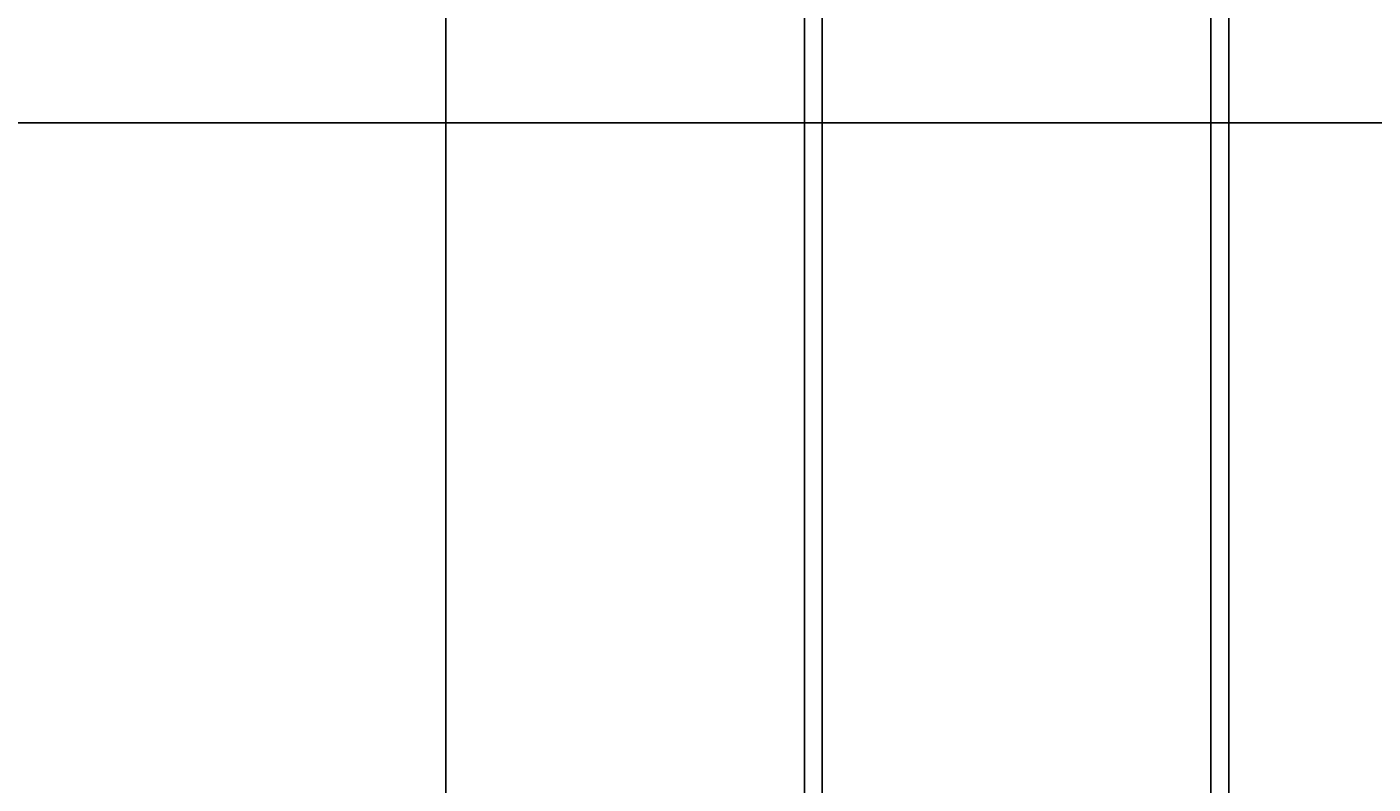
# Model space of a CAD drawing. Units: inches. Extents: x 1770 to 2988, y 1161 to 3221.
# Tile 19 of 44: x 2090 to 2289, y 2409 to 2520. Entities that reach past the tile are written whole.
import ezdxf

# ---------------------------------------------------------------- set-up
doc = ezdxf.new("R2010")
doc.units = ezdxf.units.IN
doc.layers.add('A-ANNO-DIMS', color=2, linetype='Continuous', lineweight=18)
doc.layers.add('C-PROP', color=7, linetype='Continuous', lineweight=25)
doc.styles.get("Standard").update_dxf_attribs({"font": 'arial.ttf'})
doc.dimstyles.get("Standard").update_dxf_attribs({"dimtxt": 0.18, "dimasz": 0.18, "dimexe": 0.18, "dimexo": 0.0625, "dimgap": 0.09, "dimtad": 0, "dimtih": 1, "dimtoh": 1, "dimdec": 4, "dimzin": 0, "dimdsep": 46, "dimtxsty": 'Standard', "dimcen": 0.09, "dimadec": 0, "dimazin": 0, "dimtfac": 1, "dimtdec": 4, "dimtofl": 0, "dimtmove": 0, "dimatfit": 3, "dimfxl": 1, "dimtolj": 1, "dimtzin": 0, "dimarcsym": 0})

# ---------------------------------------------------------------- blocks, each defined once
blk = doc.blocks.new('*D56')
at = {"layer": 'A-ANNO-DIMS', "color": 0, "lineweight": -2, "transparency": 16777216}
for p, q in [((1971.53, 2506.34), (1971.53, 2570.7)), ((1971.71, 2570.52), (2386.59, 2570.52)), ((2802.26, 2570.52), (2387.38, 2570.52)), ((2802.44, 2506.34), (2802.44, 2570.7))]:
    blk.add_line(p, q, dxfattribs=at)
at = {"layer": 'A-ANNO-DIMS', "color": 0, "transparency": 16777216}
for points in [[(1971.71, 2570.55), (1971.71, 2570.49), (1971.53, 2570.52)], [(2802.26, 2570.55), (2802.26, 2570.49), (2802.44, 2570.52)]]:
    blk.add_solid(points, dxfattribs=at)
at = {"layer": 'Defpoints', "color": 0, "transparency": 16777216}
for p in [(2802.44, 2570.52), (1971.53, 2506.27), (2802.44, 2506.27)]:
    blk.add_point(p, dxfattribs=at)
at = {"layer": 'A-ANNO-DIMS', "color": 0, "transparency": 16777216, "insert": (2386.99, 2570.52), "char_height": 0.18, "attachment_point": 5}
blk.add_mtext('\\A1;830.9', dxfattribs=at)
blk = doc.blocks.new('*D64')
at = {"layer": 'A-ANNO-DIMS', "color": 0, "lineweight": -2, "transparency": 16777216}
for p, q in [((2151.7, 2376.76), (2151.7, 2570.7)), ((2151.88, 2570.52), (2179.09, 2570.52)), ((2207.1, 2570.52), (2179.88, 2570.52)), ((2207.28, 2376.76), (2207.28, 2570.7))]:
    blk.add_line(p, q, dxfattribs=at)
at = {"layer": 'A-ANNO-DIMS', "color": 0, "transparency": 16777216}
for points in [[(2151.88, 2570.55), (2151.88, 2570.49), (2151.7, 2570.52)], [(2207.1, 2570.55), (2207.1, 2570.49), (2207.28, 2570.52)]]:
    blk.add_solid(points, dxfattribs=at)
at = {"layer": 'Defpoints', "color": 0, "transparency": 16777216}
for p in [(2207.28, 2570.52), (2151.7, 2376.7), (2207.28, 2376.7)]:
    blk.add_point(p, dxfattribs=at)
at = {"layer": 'A-ANNO-DIMS', "color": 0, "transparency": 16777216, "insert": (2179.49, 2570.52), "char_height": 0.18, "attachment_point": 5}
blk.add_mtext('\\A1;55.58', dxfattribs=at)
blk = doc.blocks.new('*D65')
at = {"layer": 'A-ANNO-DIMS', "color": 0, "lineweight": -2, "transparency": 16777216}
for p, q in [((2267.28, 2376.76), (2267.28, 2570.7)), ((2267.46, 2570.52), (2320.24, 2570.52)), ((2373.79, 2570.52), (2321.01, 2570.52)), ((2373.97, 2376.76), (2373.97, 2570.7))]:
    blk.add_line(p, q, dxfattribs=at)
at = {"layer": 'A-ANNO-DIMS', "color": 0, "transparency": 16777216}
for points in [[(2267.46, 2570.55), (2267.46, 2570.49), (2267.28, 2570.52)], [(2373.79, 2570.55), (2373.79, 2570.49), (2373.97, 2570.52)]]:
    blk.add_solid(points, dxfattribs=at)
at = {"layer": 'Defpoints', "color": 0, "transparency": 16777216}
for p in [(2373.97, 2570.52), (2267.28, 2376.7), (2373.97, 2376.7)]:
    blk.add_point(p, dxfattribs=at)
at = {"layer": 'A-ANNO-DIMS', "color": 0, "transparency": 16777216, "insert": (2320.62, 2570.52), "char_height": 0.18, "attachment_point": 5}
blk.add_mtext('\\A1;106.7', dxfattribs=at)
blk = doc.blocks.new('*D79')
at = {"layer": 'A-ANNO-DIMS', "color": 0, "lineweight": -2, "transparency": 16777216}
for p, q in [((2151.7, 1610.26), (2151.7, 2570.7)), ((2151.88, 2570.52), (2177.78, 2570.52)), ((2204.48, 2570.52), (2178.57, 2570.52)), ((2204.66, 1610.26), (2204.66, 2570.7))]:
    blk.add_line(p, q, dxfattribs=at)
at = {"layer": 'A-ANNO-DIMS', "color": 0, "transparency": 16777216}
for points in [[(2151.88, 2570.55), (2151.88, 2570.49), (2151.7, 2570.52)], [(2204.48, 2570.55), (2204.48, 2570.49), (2204.66, 2570.52)]]:
    blk.add_solid(points, dxfattribs=at)
at = {"layer": 'Defpoints', "color": 0, "transparency": 16777216}
for p in [(2204.66, 2570.52), (2151.7, 1610.2), (2204.66, 1610.2)]:
    blk.add_point(p, dxfattribs=at)
at = {"layer": 'A-ANNO-DIMS', "color": 0, "transparency": 16777216, "insert": (2178.18, 2570.52), "char_height": 0.18, "attachment_point": 5}
blk.add_mtext('\\A1;52.96', dxfattribs=at)
blk = doc.blocks.new('*D80')
at = {"layer": 'A-ANNO-DIMS', "color": 0, "lineweight": -2, "transparency": 16777216}
for p, q in [((2264.66, 1610.26), (2264.66, 2570.7)), ((2264.84, 2570.52), (2314.14, 2570.52)), ((2364.23, 2570.52), (2314.93, 2570.52)), ((2364.41, 1610.26), (2364.41, 2570.7))]:
    blk.add_line(p, q, dxfattribs=at)
at = {"layer": 'A-ANNO-DIMS', "color": 0, "transparency": 16777216}
for points in [[(2264.84, 2570.55), (2264.84, 2570.49), (2264.66, 2570.52)], [(2364.23, 2570.55), (2364.23, 2570.49), (2364.41, 2570.52)]]:
    blk.add_solid(points, dxfattribs=at)
at = {"layer": 'Defpoints', "color": 0, "transparency": 16777216}
for p in [(2364.41, 2570.52), (2264.66, 1610.2), (2364.41, 1610.2)]:
    blk.add_point(p, dxfattribs=at)
at = {"layer": 'A-ANNO-DIMS', "color": 0, "transparency": 16777216, "insert": (2314.53, 2570.52), "char_height": 0.18, "attachment_point": 5}
blk.add_mtext('\\A1;99.76', dxfattribs=at)

msp = doc.modelspace()

# ---------------------------------------------------------------- linework, layer by layer
at = {"layer": 'C-PROP'}
msp.add_lwpolyline([(1971.5344, 2506.2747), (2802.4374, 2506.2747), (2802.4374, 1323.5288), (1971.5344, 1323.5288)], close=True, dxfattribs=at)

# ---------------------------------------------------------------- dimensions: what is measured, and where the dimension line sits
at = {"layer": 'A-ANNO-DIMS'}
for base, p1, p2, override, picture, middle in [((2802.4374, 2570.5247), (1971.5344, 2506.2747), (2802.4374, 2506.2747), {"dimdec": 1, "dimlfac": 1, "dimrnd": 0, "dimzin": 0, "dimdsep": 46, "dimlunit": 2}, '*D56', (2386.9859, 2570.5247)), ((2207.2776, 2570.5247), (2151.696, 2376.7021), (2207.2776, 2376.7021), {"dimdec": 2, "dimlfac": 1, "dimrnd": 0, "dimzin": 0, "dimdsep": 46, "dimlunit": 2}, '*D64', (2179.4868, 2570.5247)), ((2204.6568, 2570.5247), (2151.696, 1610.2021), (2204.6568, 1610.2021), {"dimdec": 2, "dimlfac": 1, "dimrnd": 0, "dimzin": 0, "dimdsep": 46, "dimlunit": 2}, '*D79', (2178.1764, 2570.5247)), ((2364.4122, 2570.5247), (2264.6568, 1610.2021), (2364.4122, 1610.2021), {"dimdec": 2, "dimlfac": 1, "dimrnd": 0, "dimzin": 0, "dimdsep": 46, "dimlunit": 2}, '*D80', (2314.5345, 2570.5247)), ((2373.9714, 2570.5247), (2267.2776, 2376.7021), (2373.9714, 2376.7021), {"dimdec": 1, "dimlfac": 1, "dimrnd": 0, "dimzin": 0, "dimdsep": 46, "dimlunit": 2}, '*D65', (2320.6245, 2570.5247))]:
    dim = msp.add_linear_dim(base=base, p1=p1, p2=p2, dimstyle='Standard', override=override, dxfattribs=at)
    dim.commit()
    dim.dimension.update_dxf_attribs({"geometry": picture, "text_midpoint": middle})

doc.saveas('drawing.dxf')
